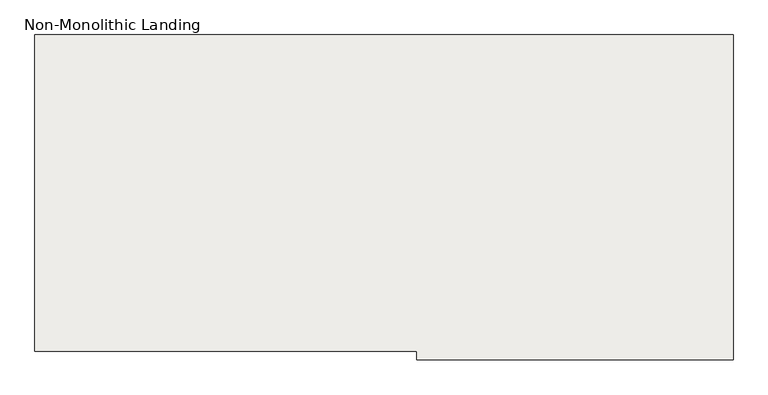
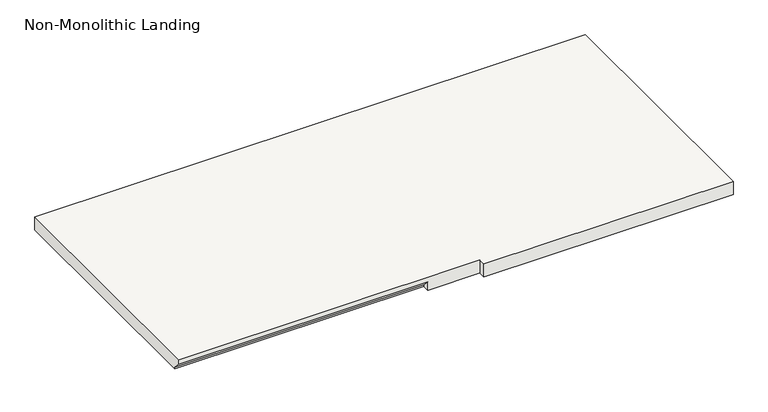
"""IFC4 building model written with IfcOpenShell, lengths in millimetres: slab geometry, Non-Monolithic Landing."""

from ifc_helpers import new_model, si_unit, origin, place, context, project, spatial, faceted_brep, source, transform, mapped, element, save


def non_monolithic_landing_2b816123(model_context):
    return source(origin(), model_context, "Body", "Brep", [
        faceted_brep([(-12643.368339, 8412.443496, 2190.75), (-12643.368339, 8437.843496, 2165.35), (-11728.968339, 8437.843496, 2165.35), (-11728.968339, 8412.443496, 2190.75), (-11538.468339, 8412.443496, 2209.8), (-11538.468339, 8387.043496, 2209.8), (-10624.068339, 8387.043496, 2209.8), (-10624.068339, 8412.443496, 2209.8), (-10624.068339, 9326.843496, 2209.8), (-12643.368339, 9326.843496, 2209.8), (-12643.368339, 8412.443496, 2209.8), (-11728.968339, 8437.843496, 2159.0), (-12643.368339, 8437.843496, 2159.0), (-12643.368339, 9326.843496, 2159.0), (-10624.068339, 9326.843496, 2159.0), (-10624.068339, 8412.443496, 2159.0), (-10624.068339, 8387.043496, 2159.0), (-11538.468339, 8387.043496, 2159.0), (-11538.468339, 8412.443496, 2159.0), (-11728.968339, 8412.443496, 2159.0)], [[[0, 1, 2, 3]], [[4, 5, 6, 7, 8, 9, 10]], [[11, 12, 13, 14, 15, 16, 17, 18, 19]], [[12, 11, 2, 1]], [[11, 19, 3, 2]], [[4, 10, 0, 3, 19, 18]], [[5, 4, 18, 17]], [[6, 5, 17, 16]], [[7, 6, 16, 15]], [[8, 7, 15, 14]], [[9, 8, 14, 13]], [[10, 9, 13, 12, 1, 0]]]),
    ])


if __name__ == "__main__":
    model = new_model("IFC4")
    model_context = context("Model", 3, world=origin())
    ifc_project = project(units=[si_unit("LENGTHUNIT", "METRE", prefix="MILLI")], contexts=[model_context])
    site = spatial("IfcSite", under=ifc_project)
    building = spatial("IfcBuilding", under=site)
    placement = place(None, origin())
    non_monolithic_landing_shape = non_monolithic_landing_2b816123(model_context)
    element("IfcSlab", 1, ObjectType="Non-Monolithic Landing", at=placement, inside=building, context=model_context, shape_type="MappedRepresentation", body=[
        mapped(non_monolithic_landing_shape, transform((0.0, 0.0, 0.0), x_axis=(1.0, 0.0, 0.0), y_axis=(0.0, 1.0, 0.0), z_axis=(0.0, 0.0, 1.0))),
    ])
    save(model, "model.ifc")
